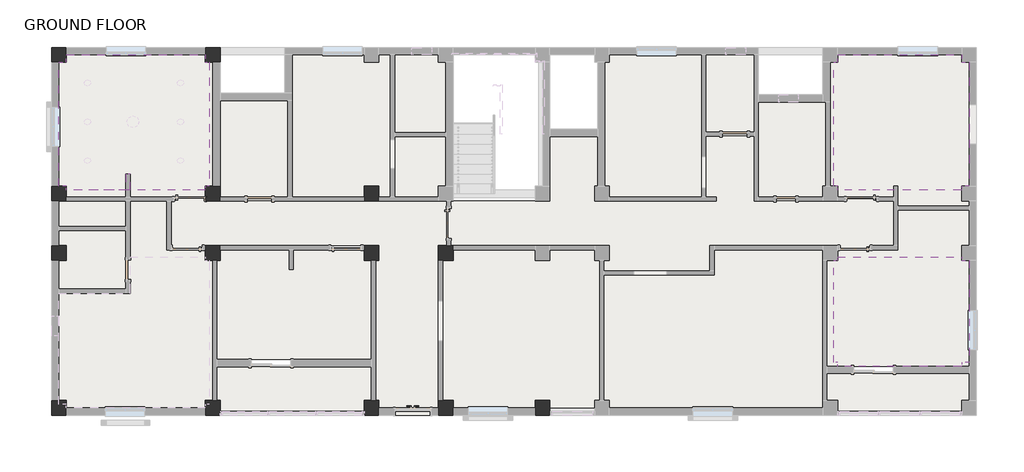
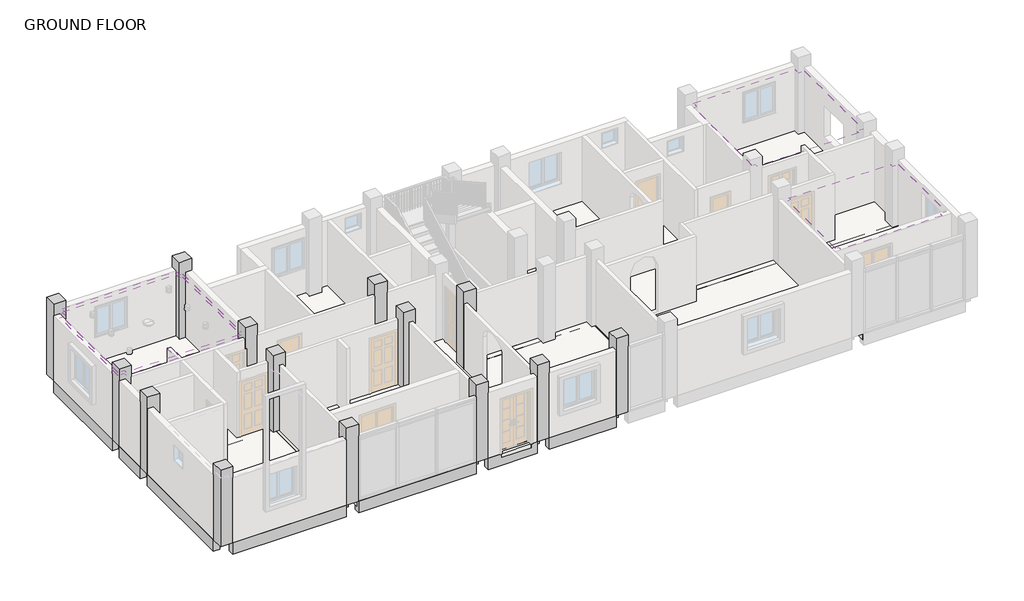
# One storey, part 3 of 5: 21 beams, 14 columns, 4 coverings, 4 slabs.
"""IFC4 building model written with IfcOpenShell, lengths in millimetres."""

from ifc_helpers import new_model, si_unit, point, frame, frame_2d, origin, place, context, project, spatial, polyline, circle_curve, trimmed, segment, composite_curve, outline, extrude, faceted_brep, element, save

model = new_model("IFC4")

# Units and contexts
model_context = context("Model", 3, world=origin())
ifc_project = project(units=[si_unit("LENGTHUNIT", "METRE", prefix="MILLI")], contexts=[model_context])

# Site, building, storey
site = spatial("IfcSite", under=ifc_project)
building = spatial("IfcBuilding", under=site)
storey = spatial("IfcBuildingStorey", under=building, Name="GROUND FLOOR", Elevation=304.8)

# Beams
placement = place(None, origin())
element("IfcBeam", 1, ObjectType="Concrete-Rectangular Beam : 9\" X 18\" BEAM", at=placement, inside=storey, context=model_context, shape_type="SweptSolid", body=[
    extrude(outline(polyline([(-10649.5456086, -10887.8679047), (-10649.5456086, -11116.4679047), (-14916.7456086, -11116.4679047), (-14916.7456086, -10887.8679047), (-10649.5456086, -10887.8679047)])), frame((0.0, 0.0, -152.4), z_axis=(0.0, 0.0, 1.0), x_axis=(1.0, 0.0, 0.0)), (0.0, 0.0, 1.0), 457.2),
])
element("IfcBeam", 2, ObjectType="Concrete-Rectangular Beam : 9\" X 18\" BEAM", at=placement, inside=storey, context=model_context, shape_type="SweptSolid", body=[
    extrude(outline(polyline([(-5772.7456086, -10887.8679047), (-5772.7456086, -11116.4679047), (-10192.3456086, -11116.4679047), (-10192.3456086, -10887.8679047), (-5772.7456086, -10887.8679047)])), frame((0.0, 0.0, -152.4), z_axis=(0.0, 0.0, 1.0), x_axis=(1.0, 0.0, 0.0)), (0.0, 0.0, 1.0), 457.2),
])
element("IfcBeam", 3, ObjectType="Concrete-Rectangular Beam : 9\" X 18\" BEAM", at=placement, inside=storey, context=model_context, shape_type="Brep", body=[
    faceted_brep([(-5315.5456086, -10887.8679047, 304.8), (-5315.5456086, -11116.4679047, 304.8), (-4807.5456086, -11116.4679047, 304.8), (-4807.5456086, -10887.8679047, 304.8), (-5315.5456086, -11116.4679047, -152.4), (-3486.7456086, -11116.4679047, -152.4), (-3486.7456086, -11116.4679047, 304.8), (-3715.3456086, -11116.4679047, 304.8), (-3715.3456086, -11116.4679047, 152.4), (-4807.5456086, -11116.4679047, 152.4), (-5315.5456086, -10887.8679047, -152.4), (-3486.7456086, -10887.8679047, -152.4), (-5315.5456086, -10887.8679047, 152.4), (-4807.5456086, -10887.8679047, 152.4), (-3715.3456086, -10887.8679047, 152.4), (-3715.3456086, -10887.8679047, 304.8), (-3486.7456086, -10887.8679047, 304.8), (-3486.7456086, -10887.8679047, 152.4)], [[[0, 1, 2, 3]], [[4, 5, 6, 7, 8, 9, 2, 1]], [[5, 4, 10, 11]], [[11, 10, 12, 0, 3, 13, 14, 15, 16, 17]], [[16, 6, 5, 11, 17]], [[10, 4, 1, 0, 12]], [[8, 14, 13, 9]], [[14, 8, 7, 15]], [[9, 13, 3, 2]], [[6, 16, 15, 7]]]),
])
element("IfcBeam", 4, ObjectType="Concrete-Rectangular Beam : 9\" X 18\" BEAM", at=placement, inside=storey, context=model_context, shape_type="SweptSolid", body=[
    extrude(outline(polyline([(-518.4083398, -10887.8679047), (-518.4083398, -11116.4679047), (-3029.5456086, -11116.4679047), (-3029.5456086, -10887.8679047), (-518.4083398, -10887.8679047)])), frame((0.0, 0.0, -152.4), z_axis=(0.0, 0.0, 1.0), x_axis=(1.0, 0.0, 0.0)), (0.0, 0.0, 1.0), 457.2),
])
element("IfcBeam", 5, ObjectType="Concrete-Rectangular Beam : 9\" X 18\" BEAM", at=placement, inside=storey, context=model_context, shape_type="SweptSolid", body=[
    extrude(outline(polyline([(-15145.3456086, -4072.3794704), (-15373.9456086, -4072.3794704), (-15373.9456086, -262.3794704), (-15145.3456086, -262.3794704), (-15145.3456086, -4072.3794704)])), frame((0.0, 0.0, -152.4), z_axis=(0.0, 0.0, 1.0), x_axis=(1.0, 0.0, 0.0)), (0.0, 0.0, 1.0), 457.2),
])
element("IfcBeam", 6, ObjectType="Concrete-Rectangular Beam : 9\" X 18\" BEAM", at=placement, inside=storey, context=model_context, shape_type="SweptSolid", body=[
    extrude(outline(polyline([(-15145.3456086, -5901.1794704), (-15373.9456086, -5901.1794704), (-15373.9456086, -4529.5794704), (-15145.3456086, -4529.5794704), (-15145.3456086, -5901.1794704)])), frame((0.0, 0.0, -152.4), z_axis=(0.0, 0.0, 1.0), x_axis=(1.0, 0.0, 0.0)), (0.0, 0.0, 1.0), 457.2),
])
element("IfcBeam", 7, ObjectType="Concrete-Rectangular Beam : 9\" X 18\" BEAM", at=placement, inside=storey, context=model_context, shape_type="SweptSolid", body=[
    extrude(outline(polyline([(-15145.3456086, -10659.2679047), (-15373.9456086, -10659.2679047), (-15373.9456086, -6358.3794704), (-15145.3456086, -6358.3794704), (-15145.3456086, -10659.2679047)])), frame((0.0, 0.0, -152.4), z_axis=(0.0, 0.0, 1.0), x_axis=(1.0, 0.0, 0.0)), (0.0, 0.0, 1.0), 457.2),
])
element("IfcBeam", 8, ObjectType="Concrete-Rectangular Beam : 9\" X 18\" BEAM", at=placement, inside=storey, context=model_context, shape_type="Brep", body=[
    faceted_brep([(-10649.5456086, -4186.6794704, 304.8), (-14916.7456086, -4186.6794704, 304.8), (-14916.7456086, -4415.2794704, 304.8), (-11589.3456086, -4415.2794704, 304.8), (-11589.3456086, -4402.5794704, 304.8), (-10674.9456086, -4402.5794704, 304.8), (-10674.9456086, -4415.2794704, 304.8), (-10649.5456086, -4415.2794704, 304.8), (-14916.7456086, -4415.2794704, -152.4), (-10649.5456086, -4415.2794704, -152.4), (-10674.9456086, -4415.2794704, 152.4), (-11589.3456086, -4415.2794704, 152.4), (-14916.7456086, -4186.6794704, -152.4), (-10649.5456086, -4186.6794704, -152.4), (-10674.9456086, -4402.5794704, 152.4), (-11589.3456086, -4402.5794704, 152.4)], [[[0, 1, 2, 3, 4, 5, 6, 7]], [[8, 9, 7, 6, 10, 11, 3, 2]], [[9, 8, 12, 13]], [[1, 0, 13, 12]], [[1, 12, 8, 2]], [[0, 7, 9, 13]], [[14, 15, 11, 10]], [[15, 4, 3, 11]], [[15, 14, 5, 4]], [[5, 14, 10, 6]]]),
])
element("IfcBeam", 9, ObjectType="Concrete-Rectangular Beam : 9\" X 18\" BEAM", at=placement, inside=storey, context=model_context, shape_type="SweptSolid", body=[
    extrude(outline(polyline([(-5772.7456086, -4186.6794704), (-5772.7456086, -4415.2794704), (-10192.3456086, -4415.2794704), (-10192.3456086, -4186.6794704), (-5772.7456086, -4186.6794704)])), frame((0.0, 0.0, -152.4), z_axis=(0.0, 0.0, 1.0), x_axis=(1.0, 0.0, 0.0)), (0.0, 0.0, 1.0), 457.2),
])
element("IfcBeam", 10, ObjectType="Concrete-Rectangular Beam : 9\" X 18\" BEAM", at=placement, inside=storey, context=model_context, shape_type="SweptSolid", body=[
    extrude(outline(polyline([(-3486.7456086, -4186.6794704), (-3486.7456086, -4415.2794704), (-5315.5456086, -4415.2794704), (-5315.5456086, -4186.6794704), (-3486.7456086, -4186.6794704)])), frame((0.0, 0.0, -152.4), z_axis=(0.0, 0.0, 1.0), x_axis=(1.0, 0.0, 0.0)), (0.0, 0.0, 1.0), 457.2),
])
element("IfcBeam", 11, ObjectType="Concrete-Rectangular Beam : 9\" X 18\" BEAM", at=placement, inside=storey, context=model_context, shape_type="SweptSolid", body=[
    extrude(outline(polyline([(-10306.6456086, -4072.3794704), (-10535.2456086, -4072.3794704), (-10535.2456086, -262.3794704), (-10306.6456086, -262.3794704), (-10306.6456086, -4072.3794704)])), frame((0.0, 0.0, -152.4), z_axis=(0.0, 0.0, 1.0), x_axis=(1.0, 0.0, 0.0)), (0.0, 0.0, 1.0), 457.2),
])
element("IfcBeam", 12, ObjectType="Concrete-Rectangular Beam : 9\" X 18\" BEAM", at=placement, inside=storey, context=model_context, shape_type="SweptSolid", body=[
    extrude(outline(polyline([(-10649.5456086, -6015.4794704), (-10649.5456086, -6244.0794704), (-14916.7456086, -6244.0794704), (-14916.7456086, -6015.4794704), (-10649.5456086, -6015.4794704)])), frame((0.0, 0.0, -152.4), z_axis=(0.0, 0.0, 1.0), x_axis=(1.0, 0.0, 0.0)), (0.0, 0.0, 1.0), 457.2),
])
element("IfcBeam", 13, ObjectType="Concrete-Rectangular Beam : 9\" X 18\" BEAM", at=placement, inside=storey, context=model_context, shape_type="SweptSolid", body=[
    extrude(outline(polyline([(-5772.7456086, -6015.4794704), (-5772.7456086, -6244.0794704), (-10192.3456086, -6244.0794704), (-10192.3456086, -6015.4794704), (-5772.7456086, -6015.4794704)])), frame((0.0, 0.0, -152.4), z_axis=(0.0, 0.0, 1.0), x_axis=(1.0, 0.0, 0.0)), (0.0, 0.0, 1.0), 457.2),
])
element("IfcBeam", 14, ObjectType="Concrete-Rectangular Beam : 9\" X 18\" BEAM", at=placement, inside=storey, context=model_context, shape_type="SweptSolid", body=[
    extrude(outline(polyline([(-3486.7456086, -6244.0794704), (-5315.5456086, -6244.0794704), (-5315.5456086, -6015.4794704), (-3486.7456086, -6015.4794704), (-3486.7456086, -6244.0794704)])), frame((0.0, 0.0, -152.4), z_axis=(0.0, 0.0, 1.0), x_axis=(1.0, 0.0, 0.0)), (0.0, 0.0, 1.0), 304.8),
])
element("IfcBeam", 15, ObjectType="Concrete-Rectangular Beam : 9\" X 18\" BEAM", at=placement, inside=storey, context=model_context, shape_type="SweptSolid", body=[
    extrude(outline(polyline([(-3029.5456086, -6244.0794704), (-3029.5456086, -6015.4794704), (-518.4083398, -6015.4794704), (-518.4083398, -6244.0794704), (-3029.5456086, -6244.0794704)])), frame((0.0, 0.0, -152.4), z_axis=(0.0, 0.0, 1.0), x_axis=(1.0, 0.0, 0.0)), (0.0, 0.0, 1.0), 457.2),
])
element("IfcBeam", 16, ObjectType="Concrete-Rectangular Beam : 9\" X 18\" BEAM", at=placement, inside=storey, context=model_context, shape_type="SweptSolid", body=[
    extrude(outline(polyline([(-10535.2456086, -6358.3794704), (-10306.6456086, -6358.3794704), (-10306.6456086, -10659.2679047), (-10535.2456086, -10659.2679047), (-10535.2456086, -6358.3794704)])), frame((0.0, 0.0, -152.4), z_axis=(0.0, 0.0, 1.0), x_axis=(1.0, 0.0, 0.0)), (0.0, 0.0, 1.0), 457.2),
])
element("IfcBeam", 17, ObjectType="Concrete-Rectangular Beam : 9\" X 18\" BEAM", at=placement, inside=storey, context=model_context, shape_type="SweptSolid", body=[
    extrude(outline(polyline([(-5658.4456086, -6358.3794704), (-5429.8456086, -6358.3794704), (-5429.8456086, -10659.2679047), (-5658.4456086, -10659.2679047), (-5658.4456086, -6358.3794704)])), frame((0.0, 0.0, -152.4), z_axis=(0.0, 0.0, 1.0), x_axis=(1.0, 0.0, 0.0)), (0.0, 0.0, 1.0), 457.2),
])
element("IfcBeam", 18, ObjectType="Concrete-Rectangular Beam : 9\" X 18\" BEAM", at=placement, inside=storey, context=model_context, shape_type="SweptSolid", body=[
    extrude(outline(polyline([(-3372.4456086, -6358.3794704), (-3143.8456086, -6358.3794704), (-3143.8456086, -10659.2679047), (-3372.4456086, -10659.2679047), (-3372.4456086, -6358.3794704)])), frame((0.0, 0.0, -152.4), z_axis=(0.0, 0.0, 1.0), x_axis=(1.0, 0.0, 0.0)), (0.0, 0.0, 1.0), 457.2),
])
element("IfcBeam", 19, ObjectType="Concrete-Rectangular Beam : 9\" X 18\" BEAM", at=placement, inside=storey, context=model_context, shape_type="SweptSolid", body=[
    extrude(outline(polyline([(-404.1083398, -6358.3794704), (-175.5083398, -6358.3794704), (-175.5083398, -10659.2679047), (-404.1083398, -10659.2679047), (-404.1083398, -6358.3794704)])), frame((0.0, 0.0, -152.4), z_axis=(0.0, 0.0, 1.0), x_axis=(1.0, 0.0, 0.0)), (0.0, 0.0, 1.0), 457.2),
])
element("IfcBeam", 20, ObjectType="Concrete-Rectangular Beam : 9\" X 18\" BEAM", at=placement, inside=storey, context=model_context, shape_type="SweptSolid", body=[
    extrude(outline(polyline([(-5658.4456086, -5901.1794704), (-5658.4456086, -4529.5794704), (-5429.8456086, -4529.5794704), (-5429.8456086, -5901.1794704), (-5658.4456086, -5901.1794704)])), frame((0.0, 0.0, -152.4), z_axis=(0.0, 0.0, 1.0), x_axis=(1.0, 0.0, 0.0)), (0.0, 0.0, 1.0), 304.8),
])
element("IfcBeam", 21, ObjectType="Concrete-Rectangular Beam : 9\" X 18\" BEAM", at=placement, inside=storey, context=model_context, shape_type="SweptSolid", body=[
    extrude(outline(polyline([(-10535.2456086, -5901.1794704), (-10535.2456086, -4529.5794704), (-10306.6456086, -4529.5794704), (-10306.6456086, -5901.1794704), (-10535.2456086, -5901.1794704)])), frame((0.0, 0.0, -152.4), z_axis=(0.0, 0.0, 1.0), x_axis=(1.0, 0.0, 0.0)), (0.0, 0.0, 1.0), 304.8),
])

# Columns
element("IfcColumn", 22, ObjectType="Concrete-Rectangular-Column : COLUMN 18\" X 18\"", at=placement, inside=storey, context=model_context, shape_type="SweptSolid", body=[
    extrude(outline(polyline([(-14916.7456086, 194.8205296), (-14916.7456086, -262.3794704), (-15373.9456086, -262.3794704), (-15373.9456086, 194.8205296), (-14916.7456086, 194.8205296)])), frame((0.0, 0.0, 304.8), z_axis=(0.0, 0.0, 1.0), x_axis=(1.0, 0.0, 0.0)), (0.0, 0.0, 1.0), 3048.0),
])
element("IfcColumn", 23, ObjectType="Concrete-Rectangular-Column : COLUMN 18\" X 18\"", at=placement, inside=storey, context=model_context, shape_type="SweptSolid", body=[
    extrude(outline(polyline([(-10192.3456086, 194.8205296), (-10192.3456086, -262.3794704), (-10649.5456086, -262.3794704), (-10649.5456086, 194.8205296), (-10192.3456086, 194.8205296)])), frame((0.0, 0.0, 304.8), z_axis=(0.0, 0.0, 1.0), x_axis=(1.0, 0.0, 0.0)), (0.0, 0.0, 1.0), 3048.0),
])
element("IfcColumn", 24, ObjectType="Concrete-Rectangular-Column : COLUMN 18\" X 18\"", at=placement, inside=storey, context=model_context, shape_type="SweptSolid", body=[
    extrude(outline(polyline([(-61.2083398, -10659.2679047), (-61.2083398, -11116.4679047), (-518.4083398, -11116.4679047), (-518.4083398, -10659.2679047), (-61.2083398, -10659.2679047)])), frame((0.0, 0.0, 304.8), z_axis=(0.0, 0.0, 1.0), x_axis=(1.0, 0.0, 0.0)), (0.0, 0.0, 1.0), 3048.0),
])
element("IfcColumn", 25, ObjectType="Concrete-Rectangular-Column : COLUMN 18\" X 18\"", at=placement, inside=storey, context=model_context, shape_type="SweptSolid", body=[
    extrude(outline(polyline([(-3029.5456086, -10659.2679047), (-3029.5456086, -11116.4679047), (-3486.7456086, -11116.4679047), (-3486.7456086, -10659.2679047), (-3029.5456086, -10659.2679047)])), frame((0.0, 0.0, 304.8), z_axis=(0.0, 0.0, 1.0), x_axis=(1.0, 0.0, 0.0)), (0.0, 0.0, 1.0), 3048.0),
])
element("IfcColumn", 26, ObjectType="Concrete-Rectangular-Column : COLUMN 18\" X 18\"", at=placement, inside=storey, context=model_context, shape_type="SweptSolid", body=[
    extrude(outline(polyline([(-5315.5456086, -10659.2679047), (-5315.5456086, -11116.4679047), (-5772.7456086, -11116.4679047), (-5772.7456086, -10659.2679047), (-5315.5456086, -10659.2679047)])), frame((0.0, 0.0, 304.8), z_axis=(0.0, 0.0, 1.0), x_axis=(1.0, 0.0, 0.0)), (0.0, 0.0, 1.0), 3048.0),
])
element("IfcColumn", 27, ObjectType="Concrete-Rectangular-Column : COLUMN 18\" X 18\"", at=placement, inside=storey, context=model_context, shape_type="SweptSolid", body=[
    extrude(outline(polyline([(-10192.3456086, -10659.2679047), (-10192.3456086, -11116.4679047), (-10649.5456086, -11116.4679047), (-10649.5456086, -10659.2679047), (-10192.3456086, -10659.2679047)])), frame((0.0, 0.0, 304.8), z_axis=(0.0, 0.0, 1.0), x_axis=(1.0, 0.0, 0.0)), (0.0, 0.0, 1.0), 3048.0),
])
element("IfcColumn", 28, ObjectType="Concrete-Rectangular-Column : COLUMN 18\" X 18\"", at=placement, inside=storey, context=model_context, shape_type="SweptSolid", body=[
    extrude(outline(polyline([(-14916.7456086, -10659.2679047), (-14916.7456086, -11116.4679047), (-15373.9456086, -11116.4679047), (-15373.9456086, -10659.2679047), (-14916.7456086, -10659.2679047)])), frame((0.0, 0.0, 304.8), z_axis=(0.0, 0.0, 1.0), x_axis=(1.0, 0.0, 0.0)), (0.0, 0.0, 1.0), 3048.0),
])
element("IfcColumn", 29, ObjectType="Concrete-Rectangular-Column : COLUMN 18\" X 18\"", at=placement, inside=storey, context=model_context, shape_type="SweptSolid", body=[
    extrude(outline(polyline([(-14916.7456086, -5901.1794704), (-14916.7456086, -6358.3794704), (-15373.9456086, -6358.3794704), (-15373.9456086, -5901.1794704), (-14916.7456086, -5901.1794704)])), frame((0.0, 0.0, 304.8), z_axis=(0.0, 0.0, 1.0), x_axis=(1.0, 0.0, 0.0)), (0.0, 0.0, 1.0), 3048.0),
])
element("IfcColumn", 30, ObjectType="Concrete-Rectangular-Column : COLUMN 18\" X 18\"", at=placement, inside=storey, context=model_context, shape_type="SweptSolid", body=[
    extrude(outline(polyline([(-14916.7456086, -4072.3794704), (-14916.7456086, -4529.5794704), (-15373.9456086, -4529.5794704), (-15373.9456086, -4072.3794704), (-14916.7456086, -4072.3794704)])), frame((0.0, 0.0, 304.8), z_axis=(0.0, 0.0, 1.0), x_axis=(1.0, 0.0, 0.0)), (0.0, 0.0, 1.0), 3048.0),
])
element("IfcColumn", 31, ObjectType="Concrete-Rectangular-Column : COLUMN 18\" X 18\"", at=placement, inside=storey, context=model_context, shape_type="SweptSolid", body=[
    extrude(outline(polyline([(-10192.3456086, -4072.3794704), (-10192.3456086, -4529.5794704), (-10649.5456086, -4529.5794704), (-10649.5456086, -4072.3794704), (-10192.3456086, -4072.3794704)])), frame((0.0, 0.0, 304.8), z_axis=(0.0, 0.0, 1.0), x_axis=(1.0, 0.0, 0.0)), (0.0, 0.0, 1.0), 3048.0),
])
element("IfcColumn", 32, ObjectType="Concrete-Rectangular-Column : COLUMN 18\" X 18\"", at=placement, inside=storey, context=model_context, shape_type="SweptSolid", body=[
    extrude(outline(polyline([(-5315.5456086, -4072.3794704), (-5315.5456086, -4529.5794704), (-5772.7456086, -4529.5794704), (-5772.7456086, -4072.3794704), (-5315.5456086, -4072.3794704)])), frame((0.0, 0.0, 304.8), z_axis=(0.0, 0.0, 1.0), x_axis=(1.0, 0.0, 0.0)), (0.0, 0.0, 1.0), 3048.0),
])
element("IfcColumn", 33, ObjectType="Concrete-Rectangular-Column : COLUMN 18\" X 18\"", at=placement, inside=storey, context=model_context, shape_type="SweptSolid", body=[
    extrude(outline(polyline([(-3029.5456086, -5901.1794704), (-3029.5456086, -6358.3794704), (-3486.7456086, -6358.3794704), (-3486.7456086, -5901.1794704), (-3029.5456086, -5901.1794704)])), frame((0.0, 0.0, 304.8), z_axis=(0.0, 0.0, 1.0), x_axis=(1.0, 0.0, 0.0)), (0.0, 0.0, 1.0), 3048.0),
])
element("IfcColumn", 34, ObjectType="Concrete-Rectangular-Column : COLUMN 18\" X 18\"", at=placement, inside=storey, context=model_context, shape_type="SweptSolid", body=[
    extrude(outline(polyline([(-5315.5456086, -5901.1794704), (-5315.5456086, -6358.3794704), (-5772.7456086, -6358.3794704), (-5772.7456086, -5901.1794704), (-5315.5456086, -5901.1794704)])), frame((0.0, 0.0, 304.8), z_axis=(0.0, 0.0, 1.0), x_axis=(1.0, 0.0, 0.0)), (0.0, 0.0, 1.0), 3048.0),
])
element("IfcColumn", 35, ObjectType="Concrete-Rectangular-Column : COLUMN 18\" X 18\"", at=placement, inside=storey, context=model_context, shape_type="SweptSolid", body=[
    extrude(outline(polyline([(-10192.3456086, -5901.1794704), (-10192.3456086, -6358.3794704), (-10649.5456086, -6358.3794704), (-10649.5456086, -5901.1794704), (-10192.3456086, -5901.1794704)])), frame((0.0, 0.0, 304.8), z_axis=(0.0, 0.0, 1.0), x_axis=(1.0, 0.0, 0.0)), (0.0, 0.0, 1.0), 3048.0),
])

# Coverings
element("IfcCovering", 36, ObjectType="GWB on Mtl. Stud", at=placement, inside=storey, context=model_context, shape_type="SweptSolid", body=[
    extrude(outline(polyline([(-14916.7456086, -262.3794704), (-14916.7456086, -33.7794704), (-10649.5456086, -33.7794704), (-10649.5456086, -262.3794704), (-10535.2456086, -262.3794704), (-10535.2456086, -4072.3794704), (-10649.5456086, -4072.3794704), (-10649.5456086, -4186.6794704), (-12959.7401855, -4186.6794704), (-12959.7401855, -3705.5659448), (-13086.7401855, -3705.5659448), (-13086.7401855, -4186.6794704), (-14916.7456086, -4186.6794704), (-14916.7456086, -4072.3794704), (-15145.3456086, -4072.3794704), (-15145.3456086, -262.3794704), (-14916.7456086, -262.3794704)]), holes=[composite_curve([segment(trimmed(circle_curve(frame_2d((-14269.0456086, -897.3794704)), 76.2), [point((-14345.2456086, -897.3794704))], [point((-14192.8456086, -897.3794704))], True, "CARTESIAN"), True, "CONTINUOUS"), segment(trimmed(circle_curve(frame_2d((-14269.0456086, -897.3794704)), 76.2), [point((-14192.8456086, -897.3794704))], [point((-14345.2456086, -897.3794704))], True, "CARTESIAN"), True, "CONTINUOUS")], self_intersect=False), composite_curve([segment(trimmed(circle_curve(frame_2d((-14269.0456086, -3284.9794704)), 76.2), [point((-14345.2456086, -3284.9794704))], [point((-14192.8456086, -3284.9794704))], True, "CARTESIAN"), True, "CONTINUOUS"), segment(trimmed(circle_curve(frame_2d((-14269.0456086, -3284.9794704)), 76.2), [point((-14192.8456086, -3284.9794704))], [point((-14345.2456086, -3284.9794704))], True, "CARTESIAN"), True, "CONTINUOUS")], self_intersect=False), composite_curve([segment(trimmed(circle_curve(frame_2d((-14269.0456086, -2091.1794704)), 76.2), [point((-14345.2456086, -2091.1794704))], [point((-14192.8456086, -2091.1794704))], True, "CARTESIAN"), True, "CONTINUOUS"), segment(trimmed(circle_curve(frame_2d((-14269.0456086, -2091.1794704)), 76.2), [point((-14192.8456086, -2091.1794704))], [point((-14345.2456086, -2091.1794704))], True, "CARTESIAN"), True, "CONTINUOUS")], self_intersect=False), composite_curve([segment(trimmed(circle_curve(frame_2d((-11411.5456086, -897.3794704)), 76.2), [point((-11335.3456086, -897.3794704))], [point((-11487.7456086, -897.3794704))], True, "CARTESIAN"), True, "CONTINUOUS"), segment(trimmed(circle_curve(frame_2d((-11411.5456086, -897.3794704)), 76.2), [point((-11487.7456086, -897.3794704))], [point((-11335.3456086, -897.3794704))], True, "CARTESIAN"), True, "CONTINUOUS")], self_intersect=False), composite_curve([segment(trimmed(circle_curve(frame_2d((-11411.5456086, -3284.9794704)), 76.2), [point((-11335.3456086, -3284.9794704))], [point((-11487.7456086, -3284.9794704))], True, "CARTESIAN"), True, "CONTINUOUS"), segment(trimmed(circle_curve(frame_2d((-11411.5456086, -3284.9794704)), 76.2), [point((-11487.7456086, -3284.9794704))], [point((-11335.3456086, -3284.9794704))], True, "CARTESIAN"), True, "CONTINUOUS")], self_intersect=False), composite_curve([segment(trimmed(circle_curve(frame_2d((-11411.5456086, -2091.1794704)), 76.2), [point((-11335.3456086, -2091.1794704))], [point((-11487.7456086, -2091.1794704))], True, "CARTESIAN"), True, "CONTINUOUS"), segment(trimmed(circle_curve(frame_2d((-11411.5456086, -2091.1794704)), 76.2), [point((-11487.7456086, -2091.1794704))], [point((-11335.3456086, -2091.1794704))], True, "CARTESIAN"), True, "CONTINUOUS")], self_intersect=False)]), frame((0.0, 0.0, 2870.2), z_axis=(0.0, 0.0, 1.0), x_axis=(1.0, 0.0, 0.0)), (0.0, 0.0, 1.0), 107.95),
])
element("IfcCovering", 37, ObjectType="GWB on Mtl. Stud", at=placement, inside=storey, context=model_context, shape_type="SweptSolid", body=[
    extrude(outline(polyline([(-15145.3456086, -4072.3794704), (-15145.3456086, -262.3794704), (-14916.7456086, -262.3794704), (-14916.7456086, -33.7794704), (-10649.5456086, -33.7794704), (-10649.5456086, -262.3794704), (-10535.2456086, -262.3794704), (-10535.2456086, -4072.3794704), (-10649.5456086, -4072.3794704), (-10649.5456086, -4186.6794704), (-12959.7401855, -4186.6794704), (-14916.7456086, -4186.6794704), (-14916.7456086, -4072.3794704), (-15145.3456086, -4072.3794704)]), holes=[polyline([(-14840.5456086, -3881.8794704), (-10840.0456086, -3881.8794704), (-10840.0456086, -338.5794704), (-14840.5456086, -338.5794704), (-14840.5456086, -3881.8794704)])]), frame((0.0, 0.0, 2743.2), z_axis=(0.0, 0.0, 1.0), x_axis=(1.0, 0.0, 0.0)), (0.0, 0.0, 1.0), 107.95),
    extrude(outline(polyline([(-14688.1456086, -3729.4794704), (-14688.1456086, -490.9794704), (-10992.4456086, -490.9794704), (-10992.4456086, -3729.4794704), (-14688.1456086, -3729.4794704)]), holes=[polyline([(-11144.8456086, -643.3794704), (-14535.7456086, -643.3794704), (-14535.7456086, -3577.0794704), (-11144.8456086, -3577.0794704), (-11144.8456086, -643.3794704)])]), frame((0.0, 0.0, 2743.2), z_axis=(0.0, 0.0, 1.0), x_axis=(1.0, 0.0, 0.0)), (0.0, 0.0, 1.0), 107.95),
])
element("IfcCovering", 38, ObjectType="GWB on Mtl. Stud", at=placement, inside=storey, context=model_context, shape_type="SweptSolid", body=[
    extrude(outline(polyline([(8991.0043914, -3729.4794704), (8991.0043914, -490.9794704), (12477.1543914, -490.9794704), (12477.1543914, -3729.4794704), (8991.0043914, -3729.4794704)]), holes=[polyline([(12324.7543914, -643.3794704), (9162.4543914, -643.3794704), (9162.4543914, -3577.0794704), (12324.7543914, -3577.0794704), (12324.7543914, -643.3794704)])]), frame((0.0, 0.0, 2743.2), z_axis=(0.0, 0.0, 1.0), x_axis=(1.0, 0.0, 0.0)), (0.0, 0.0, 1.0), 107.95),
    extrude(outline(polyline([(8660.1098601, -4072.3794704), (8660.1098601, -262.3794704), (8774.4128058, -262.3794704), (8774.4128058, -33.7794704), (12584.4128058, -33.7794704), (12584.4128058, -262.3794704), (12813.0098601, -262.3794704), (12813.0098601, -4072.3794704), (12584.4128058, -4072.3794704), (12584.4128058, -4186.6794704), (10509.8598145, -4186.6794704), (8774.4128058, -4186.6794704), (8774.4128058, -4072.3794704), (8660.1098601, -4072.3794704)]), holes=[polyline([(8838.6043914, -338.5794704), (8838.6043914, -3881.8794704), (12629.5543914, -3881.8794704), (12629.5543914, -338.5794704), (8838.6043914, -338.5794704)])]), frame((0.0, 0.0, 2743.2), z_axis=(0.0, 0.0, 1.0), x_axis=(1.0, 0.0, 0.0)), (0.0, 0.0, 1.0), 107.95),
])
element("IfcCovering", 39, ObjectType="GWB on Mtl. Stud", at=placement, inside=storey, context=model_context, shape_type="SweptSolid", body=[
    extrude(outline(polyline([(8991.0043914, -9147.9642361), (8991.0043914, -6726.6794704), (12477.1543914, -6726.6794704), (12477.1543914, -9147.9642361), (8991.0043914, -9147.9642361)]), holes=[polyline([(12324.7543914, -7031.4298611), (9162.4543914, -7031.4298611), (9162.4543914, -8995.5642361), (12324.7543914, -8995.5642361), (12324.7543914, -7031.4298611)])]), frame((0.0, 0.0, 2743.2), z_axis=(0.0, 0.0, 1.0), x_axis=(1.0, 0.0, 0.0)), (0.0, 0.0, 1.0), 107.95),
    extrude(outline(polyline([(8660.1098601, -9490.8642361), (8660.1098601, -6358.3685356), (8774.4128058, -6358.3685356), (8774.4128058, -6244.0794704), (12584.4128058, -6244.0794704), (12584.4128058, -6358.3794704), (12813.0098601, -6358.3794704), (12813.0098601, -9490.8642361), (12584.4128058, -9490.8642361), (12584.4128058, -9605.1642361), (10509.8598145, -9605.1642361), (8774.4128058, -9605.1642361), (8774.4128058, -9490.8642361), (8660.1098601, -9490.8642361)]), holes=[polyline([(12629.5543914, -6498.0794704), (8838.6043914, -6498.0794704), (8838.6043914, -9300.3642361), (12629.5543914, -9300.3642361), (12629.5543914, -6498.0794704)])]), frame((0.0, 0.0, 2743.2), z_axis=(0.0, 0.0, 1.0), x_axis=(1.0, 0.0, 0.0)), (0.0, 0.0, 1.0), 107.95),
])

# Slabs
element("IfcSlab", 40, ObjectType="MARBLE FLOORING 6\"", at=placement, inside=storey, context=model_context, shape_type="SweptSolid", body=[
    extrude(outline(polyline([(-13086.7401855, -4529.5794704), (-13086.7401855, -5304.2794704), (-15145.3456086, -5304.2794704), (-15145.3456086, -4529.5794704), (-13086.7401855, -4529.5794704)])), frame((0.0, 0.0, 152.4), z_axis=(0.0, 0.0, 1.0), x_axis=(1.0, 0.0, 0.0)), (0.0, 0.0, 1.0), 152.4),
    extrude(outline(polyline([(-13086.7401855, -5431.2794704), (-13086.7401855, -6334.4659448), (-13023.2401855, -6334.4659448), (-13023.2401855, -6944.0659448), (-13086.7401855, -6944.0659448), (-13086.7401855, -7236.1659448), (-15145.3456086, -7236.1659448), (-15145.3456086, -6358.3794704), (-14916.7456086, -6358.3794704), (-14916.7456086, -5901.1794704), (-15145.3456086, -5901.1794704), (-15145.3456086, -5431.2794704), (-13086.7401855, -5431.2794704)])), frame((0.0, 0.0, 152.4), z_axis=(0.0, 0.0, 1.0), x_axis=(1.0, 0.0, 0.0)), (0.0, 0.0, 1.0), 152.4),
    extrude(outline(polyline([(-8109.5456086, -1443.4794704), (-8109.5456086, -4402.5794704), (-8603.1541526, -4402.5794704), (-8603.1541526, -4529.5794704), (-9366.8456086, -4529.5794704), (-9366.8456086, -4402.5794704), (-10192.3456086, -4402.5794704), (-10192.3456086, -1443.4794704), (-8109.5456086, -1443.4794704)])), frame((0.0, 0.0, 152.4), z_axis=(0.0, 0.0, 1.0), x_axis=(1.0, 0.0, 0.0)), (0.0, 0.0, 1.0), 152.4),
    extrude(outline(polyline([(-3486.7456086, -33.7794704), (-3486.7456086, -262.3794704), (-3258.1456086, -262.3794704), (-3258.1456086, -2421.3794704), (-4832.9456086, -2421.3794704), (-4832.9456086, -33.7794704), (-3486.7456086, -33.7794704)])), frame((0.0, 0.0, 152.4), z_axis=(0.0, 0.0, 1.0), x_axis=(1.0, 0.0, 0.0)), (0.0, 0.0, 1.0), 152.4),
    extrude(outline(polyline([(6212.5916602, -33.7794704), (6212.5916602, -2408.6794704), (5996.6916602, -2408.6794704), (5996.6916602, -2535.6794704), (5234.6916602, -2535.6794704), (5234.6916602, -2408.6794704), (4726.6916602, -2408.6794704), (4726.6916602, -33.7794704), (6212.5916602, -33.7794704)])), frame((0.0, 0.0, 152.4), z_axis=(0.0, 0.0, 1.0), x_axis=(1.0, 0.0, 0.0)), (0.0, 0.0, 1.0), 152.4),
    extrude(outline(polyline([(8418.8128058, -1481.5794704), (8418.8128058, -4072.3794704), (8317.2128058, -4072.3794704), (8317.2128058, -4402.5794704), (7495.2916602, -4402.5794704), (7495.2916602, -4529.5794704), (6885.6916602, -4529.5794704), (6885.6916602, -4402.5794704), (6339.5916602, -4402.5794704), (6339.5916602, -1481.5794704), (8418.8128058, -1481.5794704)])), frame((0.0, 0.0, 152.4), z_axis=(0.0, 0.0, 1.0), x_axis=(1.0, 0.0, 0.0)), (0.0, 0.0, 1.0), 152.4),
])
element("IfcSlab", 41, ObjectType="Wood Joist 10\" - Ceramic Tile", at=placement, inside=storey, context=model_context, shape_type="SweptSolid", body=[
    extrude(outline(polyline([(-10192.3456086, -10659.2679047), (-10293.9456086, -10659.2679047), (-10293.9456086, -9630.5679047), (-5544.1456086, -9630.5679047), (-5544.1456086, -10659.2679047), (-5772.7456086, -10659.2679047), (-5772.7456086, -10989.4679047), (-10192.3456086, -10989.4679047), (-10192.3456086, -10659.2679047)])), frame((0.0, 0.0, 31.75), z_axis=(0.0, 0.0, 1.0), x_axis=(1.0, 0.0, 0.0)), (0.0, 0.0, 1.0), 273.05),
    extrude(outline(polyline([(8444.2128058, -9833.7679047), (12813.0128058, -9833.7679047), (12813.0128058, -10659.2679047), (12584.4128058, -10659.2679047), (12584.4128058, -11052.9679047), (8774.4128058, -11052.9679047), (8774.4128058, -10659.2679047), (8444.2128058, -10659.2679047), (8444.2128058, -9833.7679047)])), frame((0.0, 0.0, 31.75), z_axis=(0.0, 0.0, 1.0), x_axis=(1.0, 0.0, 0.0)), (0.0, 0.0, 1.0), 273.05),
])
element("IfcSlab", 42, ObjectType="white MARBLE FLOORING 6\" 2", at=placement, inside=storey, context=model_context, shape_type="SweptSolid", body=[
    extrude(outline(polyline([(-12959.7401855, -4402.5794704), (-12959.7401855, -3705.5659448), (-13086.7401855, -3705.5659448), (-13086.7401855, -4402.5794704), (-14916.7456086, -4402.5794704), (-14916.7456086, -4072.3794704), (-15145.3456086, -4072.3794704), (-15145.3456086, -262.3794704), (-14916.7456086, -262.3794704), (-14916.7456086, -33.7794704), (-10649.5456086, -33.7794704), (-10649.5456086, -262.3794704), (-10420.9456086, -262.3794704), (-10420.9456086, -4072.3794704), (-10649.5456086, -4072.3794704), (-10649.5456086, -4402.5794704), (-11589.3456086, -4402.5794704), (-12959.7401855, -4402.5794704)])), frame((0.0, 0.0, 152.4), z_axis=(0.0, 0.0, 1.0), x_axis=(1.0, 0.0, 0.0)), (0.0, 0.0, 1.0), 152.4),
    extrude(outline(polyline([(-15145.3456086, -10659.2679047), (-15145.3456086, -7363.1659448), (-12959.7401855, -7363.1659448), (-12959.7401855, -6944.0659448), (-13023.2401855, -6944.0659448), (-13023.2401855, -6334.4659448), (-12959.7401855, -6334.4659448), (-12959.7401855, -4529.5794704), (-11829.4401855, -4529.5794704), (-11829.4401855, -6028.1794704), (-11690.342897, -6028.1794704), (-11690.342897, -5967.8544704), (-10750.542897, -5967.8544704), (-10750.542897, -6028.1794704), (-10649.5456086, -6028.1794704), (-10649.5456086, -6358.3794704), (-10420.9456086, -6358.3794704), (-10420.9456086, -10659.2679047), (-10649.5456086, -10659.2679047), (-10649.5456086, -10887.8679047), (-14916.7456086, -10887.8679047), (-14916.7456086, -10659.2679047), (-15145.3456086, -10659.2679047)])), frame((0.0, 0.0, 152.4), z_axis=(0.0, 0.0, 1.0), x_axis=(1.0, 0.0, 0.0)), (0.0, 0.0, 1.0), 152.4),
    extrude(outline(polyline([(-5544.1456086, -9401.9679047), (-10293.9456086, -9401.9679047), (-10293.9456086, -6358.3794704), (-10192.3456086, -6358.3794704), (-10192.3456086, -6028.1794704), (-8071.4456086, -6028.1794704), (-8071.4456086, -6637.7794704), (-7944.4456086, -6637.7794704), (-7944.4456086, -6028.1794704), (-6788.7456086, -6028.1794704), (-6788.7456086, -5967.8544704), (-5874.3456086, -5967.8544704), (-5874.3456086, -6028.1794704), (-5772.7456086, -6028.1794704), (-5772.7456086, -6358.3794704), (-5544.1456086, -6358.3794704), (-5544.1456086, -9401.9679047)])), frame((0.0, 0.0, 152.4), z_axis=(0.0, 0.0, 1.0), x_axis=(1.0, 0.0, 0.0)), (0.0, 0.0, 1.0), 152.4),
    extrude(outline(polyline([(-3029.5456086, -10659.2679047), (-3359.7456086, -10659.2679047), (-3359.7456086, -6358.3794704), (-3029.5456086, -6358.3794704), (-3029.5456086, -6028.1794704), (-518.4083398, -6028.1794704), (-518.4083398, -6358.3794704), (-61.2083398, -6358.3794704), (-61.2083398, -6028.1794704), (1310.3916602, -6028.1794704), (1310.3916602, -6358.3794704), (1462.7916602, -6358.3794704), (1462.7916602, -10659.2679047), (1310.3916602, -10659.2679047), (1310.3916602, -10887.8679047), (-61.2083398, -10887.8679047), (-61.2083398, -10659.2679047), (-518.4083398, -10659.2679047), (-518.4083398, -10887.8679047), (-3029.5456086, -10887.8679047), (-3029.5456086, -10659.2679047)])), frame((0.0, 0.0, 152.4), z_axis=(0.0, 0.0, 1.0), x_axis=(1.0, 0.0, 0.0)), (0.0, 0.0, 1.0), 152.4),
    extrude(outline(polyline([(4980.6916602, -6802.8794704), (4980.6916602, -6028.1794704), (8317.2128058, -6028.1794704), (8317.2128058, -10887.8679047), (1767.5916602, -10887.8679047), (1767.5916602, -10659.2679047), (1589.7916602, -10659.2679047), (1589.7916602, -6802.8794704), (4980.6916602, -6802.8794704)])), frame((0.0, 0.0, 152.4), z_axis=(0.0, 0.0, 1.0), x_axis=(1.0, 0.0, 0.0)), (0.0, 0.0, 1.0), 152.4),
    extrude(outline(polyline([(12813.0128058, -9605.1679047), (8444.2128058, -9605.1679047), (8444.2128058, -6358.3794704), (8774.4128058, -6358.3794704), (8774.4128058, -6028.1794704), (8850.6128058, -6028.1794704), (8850.6128058, -5967.8544704), (9765.0128058, -5967.8544704), (9765.0128058, -6028.1794704), (10628.6128058, -6028.1794704), (10628.6128058, -4808.9794704), (12813.0128058, -4808.9794704), (12813.0128058, -5901.1794704), (12584.4128058, -5901.1794704), (12584.4128058, -6358.3794704), (12813.0128058, -6358.3794704), (12813.0128058, -9605.1679047)])), frame((0.0, 0.0, 152.4), z_axis=(0.0, 0.0, 1.0), x_axis=(1.0, 0.0, 0.0)), (0.0, 0.0, 1.0), 152.4),
    extrude(outline(polyline([(12813.0128058, -4681.9794704), (10628.6128058, -4681.9794704), (10628.6128058, -4072.3794704), (10501.6128058, -4072.3794704), (10501.6128058, -4402.5794704), (9968.2128058, -4402.5794704), (9968.2128058, -4466.0794704), (9053.8128058, -4466.0794704), (9053.8128058, -4402.5794704), (8774.4128058, -4402.5794704), (8774.4128058, -4072.3794704), (8545.8128058, -4072.3794704), (8545.8128058, -262.3794704), (8774.4128058, -262.3794704), (8774.4128058, -33.7794704), (12584.4128058, -33.7794704), (12584.4128058, -262.3794704), (12813.0128058, -262.3794704), (12813.0128058, -4072.3794704), (12584.4128058, -4072.3794704), (12584.4128058, -4529.5794704), (12813.0128058, -4529.5794704), (12813.0128058, -4681.9794704)])), frame((0.0, 0.0, 152.4), z_axis=(0.0, 0.0, 1.0), x_axis=(1.0, 0.0, 0.0)), (0.0, 0.0, 1.0), 152.4),
    extrude(outline(polyline([(1767.5916602, -4072.3794704), (1627.8916602, -4072.3794704), (1627.8916602, -262.3794704), (1767.5916602, -262.3794704), (1767.5916602, -33.7794704), (4599.6916602, -33.7794704), (4599.6916602, -4402.5794704), (1767.5916602, -4402.5794704), (1767.5916602, -4072.3794704)])), frame((0.0, 0.0, 152.4), z_axis=(0.0, 0.0, 1.0), x_axis=(1.0, 0.0, 0.0)), (0.0, 0.0, 1.0), 152.4),
    extrude(outline(polyline([(-5772.7456086, -33.7794704), (-5772.7456086, -262.3794704), (-5315.5456086, -262.3794704), (-5315.5456086, -33.7794704), (-4959.9456086, -33.7794704), (-4959.9456086, -4402.5794704), (-5315.5456086, -4402.5794704), (-5315.5456086, -4072.3794704), (-5772.7456086, -4072.3794704), (-5772.7456086, -4402.5794704), (-7982.5456086, -4402.5794704), (-7982.5456086, -33.7794704), (-5772.7456086, -33.7794704)])), frame((0.0, 0.0, 152.4), z_axis=(0.0, 0.0, 1.0), x_axis=(1.0, 0.0, 0.0)), (0.0, 0.0, 1.0), 152.4),
    extrude(outline(polyline([(-4832.9456086, -4402.5794704), (-4832.9456086, -2548.3794704), (-3258.1456086, -2548.3794704), (-3258.1456086, -4072.3794704), (-3486.7456086, -4072.3794704), (-3486.7456086, -4402.5794704), (-4832.9456086, -4402.5794704)])), frame((0.0, 0.0, 152.4), z_axis=(0.0, 0.0, 1.0), x_axis=(1.0, 0.0, 0.0)), (0.0, 0.0, 1.0), 152.4),
])
element("IfcSlab", 43, ObjectType="white MARBLE FLOORING 6\" 2", at=placement, inside=storey, context=model_context, shape_type="Brep", body=[
    faceted_brep([(-11589.3456086, -4529.5794704, 152.4), (-11589.3456086, -4415.2794704, 152.4), (-11589.3456086, -4402.5794704, 152.4), (-10674.9456086, -4402.5794704, 152.4), (-10674.9456086, -4415.2794704, 152.4), (-10674.9456086, -4529.5794704, 152.4), (-10535.2456086, -4529.5794704, 152.4), (-10306.6456086, -4529.5794704, 152.4), (-9366.8456086, -4529.5794704, 152.4), (-5658.4456086, -4529.5794704, 152.4), (-5429.8456086, -4529.5794704, 152.4), (-3372.4456086, -4529.5794704, 152.4), (-3143.8456086, -4529.5794704, 152.4), (-404.1083398, -4529.5794704, 152.4), (-175.5083398, -4529.5794704, 152.4), (-61.2083398, -4529.5794704, 152.4), (-61.2083398, -4415.2794704, 152.4), (-61.2083398, -4186.6794704, 152.4), (-61.2083398, -2548.3794704, 152.4), (1399.2916602, -2548.3794704, 152.4), (1399.2916602, -4072.3794704, 152.4), (1310.3916602, -4072.3794704, 152.4), (1310.3916602, -4186.6794704, 152.4), (1310.3916602, -4415.2794704, 152.4), (1310.3916602, -4529.5794704, 152.4), (1424.6916602, -4529.5794704, 152.4), (1653.2916602, -4529.5794704, 152.4), (5044.1916602, -4529.5794704, 152.4), (5044.1916602, -4415.2794704, 152.4), (5044.1916602, -4402.5794704, 152.4), (4726.6916602, -4402.5794704, 152.4), (4726.6916602, -4186.6794704, 152.4), (4726.6916602, -2535.6794704, 152.4), (6212.5916602, -2535.6794704, 152.4), (6212.5916602, -4186.6794704, 152.4), (6212.5916602, -4415.2794704, 152.4), (6212.5916602, -4529.5794704, 152.4), (8431.5128058, -4529.5794704, 152.4), (8660.1128058, -4529.5794704, 152.4), (9053.8128058, -4529.5794704, 152.4), (9053.8128058, -4466.0794704, 152.4), (9968.2128058, -4466.0794704, 152.4), (9968.2128058, -4529.5794704, 152.4), (10501.6128058, -4529.5794704, 152.4), (10501.6128058, -5901.1794704, 152.4), (9765.0128058, -5901.1794704, 152.4), (9765.0128058, -5967.8544704, 152.4), (8850.6128058, -5967.8544704, 152.4), (8850.6128058, -5901.1794704, 152.4), (8660.1128058, -5901.1794704, 152.4), (8431.5128058, -5901.1794704, 152.4), (4853.6916602, -5901.1794704, 152.4), (4853.6916602, -6015.4794704, 152.4), (4853.6916602, -6244.0794704, 152.4), (4853.6916602, -6675.8794704, 152.4), (1653.2916602, -6675.8794704, 152.4), (1589.7916602, -6675.8794704, 152.4), (1589.7916602, -6358.3794704, 152.4), (1653.2916602, -6358.3794704, 152.4), (1767.5916602, -6358.3794704, 152.4), (1767.5916602, -6244.0794704, 152.4), (1767.5916602, -6015.4794704, 152.4), (1767.5916602, -5901.1794704, 152.4), (1653.2916602, -5901.1794704, 152.4), (1424.6916602, -5901.1794704, 152.4), (-175.5083398, -5901.1794704, 152.4), (-404.1083398, -5901.1794704, 152.4), (-3105.7456086, -5901.1794704, 152.4), (-3105.7456086, -5672.5794704, 152.4), (-3143.8456086, -5672.5794704, 152.4), (-3232.7456086, -5672.5794704, 152.4), (-3232.7456086, -5901.1794704, 152.4), (-3372.4456086, -5901.1794704, 152.4), (-3486.7456086, -5901.1794704, 152.4), (-3486.7456086, -6015.4794704, 152.4), (-3486.7456086, -6244.0794704, 152.4), (-3486.7456086, -10887.8679047, 152.4), (-3715.3456086, -10887.8679047, 152.4), (-3715.3456086, -11116.4679047, 152.4), (-4807.5456086, -11116.4679047, 152.4), (-4807.5456086, -10887.8679047, 152.4), (-5315.5456086, -10887.8679047, 152.4), (-5315.5456086, -10659.2679047, 152.4), (-5417.1456086, -10659.2679047, 152.4), (-5417.1456086, -6358.3794704, 152.4), (-5315.5456086, -6358.3794704, 152.4), (-5315.5456086, -6244.0794704, 152.4), (-5315.5456086, -6015.4794704, 152.4), (-5315.5456086, -5901.1794704, 152.4), (-5429.8456086, -5901.1794704, 152.4), (-5658.4456086, -5901.1794704, 152.4), (-10306.6456086, -5901.1794704, 152.4), (-10535.2456086, -5901.1794704, 152.4), (-10750.542897, -5901.1794704, 152.4), (-10750.542897, -5967.8544704, 152.4), (-11664.942897, -5967.8544704, 152.4), (-11664.942897, -5901.1794704, 152.4), (-11702.4401855, -5901.1794704, 152.4), (-11702.4401855, -4529.5794704, 152.4), (-11589.3456086, -4529.5794704, 304.8), (-11702.4401855, -4529.5794704, 304.8), (-11702.4401855, -5901.1794704, 304.8), (-11664.942897, -5901.1794704, 304.8), (-11664.942897, -5967.8544704, 304.8), (-10750.542897, -5967.8544704, 304.8), (-10750.542897, -5901.1794704, 304.8), (-10649.5456086, -5901.1794704, 304.8), (-10192.3456086, -5901.1794704, 304.8), (-5772.7456086, -5901.1794704, 304.8), (-5315.5456086, -5901.1794704, 304.8), (-5315.5456086, -6358.3794704, 304.8), (-5417.1456086, -6358.3794704, 304.8), (-5417.1456086, -10659.2679047, 304.8), (-5315.5456086, -10659.2679047, 304.8), (-5315.5456086, -10887.8679047, 304.8), (-4807.5456086, -10887.8679047, 304.8), (-4807.5456086, -11116.4679047, 304.8), (-3715.3456086, -11116.4679047, 304.8), (-3715.3456086, -10887.8679047, 304.8), (-3486.7456086, -10887.8679047, 304.8), (-3486.7456086, -10659.2679047, 304.8), (-3486.7456086, -6358.3794704, 304.8), (-3486.7456086, -5901.1794704, 304.8), (-3232.7456086, -5901.1794704, 304.8), (-3232.7456086, -5672.5794704, 304.8), (-3143.8456086, -5672.5794704, 304.8), (-3105.7456086, -5672.5794704, 304.8), (-3105.7456086, -5901.1794704, 304.8), (-3029.5456086, -5901.1794704, 304.8), (-518.4083398, -5901.1794704, 304.8), (-61.2083398, -5901.1794704, 304.8), (1310.3916602, -5901.1794704, 304.8), (1767.5916602, -5901.1794704, 304.8), (1767.5916602, -6358.3794704, 304.8), (1589.7916602, -6358.3794704, 304.8), (1589.7916602, -6675.8794704, 304.8), (1653.2916602, -6675.8794704, 304.8), (4853.6916602, -6675.8794704, 304.8), (4853.6916602, -6244.0794704, 304.8), (4853.6916602, -6015.4794704, 304.8), (4853.6916602, -5901.1794704, 304.8), (8317.2128058, -5901.1794704, 304.8), (8774.4128058, -5901.1794704, 304.8), (8850.6128058, -5901.1794704, 304.8), (8850.6128058, -5967.8544704, 304.8), (9765.0128058, -5967.8544704, 304.8), (9765.0128058, -5901.1794704, 304.8), (10501.6128058, -5901.1794704, 304.8), (10501.6128058, -4529.5794704, 304.8), (9968.2128058, -4529.5794704, 304.8), (9968.2128058, -4466.0794704, 304.8), (9053.8128058, -4466.0794704, 304.8), (9053.8128058, -4529.5794704, 304.8), (8774.4128058, -4529.5794704, 304.8), (8317.2128058, -4529.5794704, 304.8), (6212.5916602, -4529.5794704, 304.8), (6212.5916602, -4415.2794704, 304.8), (6212.5916602, -4186.6794704, 304.8), (6212.5916602, -2535.6794704, 304.8), (4726.6916602, -2535.6794704, 304.8), (4726.6916602, -4186.6794704, 304.8), (4726.6916602, -4402.5794704, 304.8), (5044.1916602, -4402.5794704, 304.8), (5044.1916602, -4415.2794704, 304.8), (5044.1916602, -4529.5794704, 304.8), (1767.5916602, -4529.5794704, 304.8), (1310.3916602, -4529.5794704, 304.8), (1310.3916602, -4072.3794704, 304.8), (1399.2916602, -4072.3794704, 304.8), (1399.2916602, -2548.3794704, 304.8), (-61.2083398, -2548.3794704, 304.8), (-61.2083398, -4072.3794704, 304.8), (-61.2083398, -4529.5794704, 304.8), (-518.4083398, -4529.5794704, 304.8), (-3029.5456086, -4529.5794704, 304.8), (-3486.7456086, -4529.5794704, 304.8), (-5315.5456086, -4529.5794704, 304.8), (-5772.7456086, -4529.5794704, 304.8), (-9366.8456086, -4529.5794704, 304.8), (-10192.3456086, -4529.5794704, 304.8), (-10649.5456086, -4529.5794704, 304.8), (-10674.9456086, -4529.5794704, 304.8), (-10674.9456086, -4415.2794704, 304.8), (-10674.9456086, -4402.5794704, 304.8), (-11589.3456086, -4402.5794704, 304.8), (-11589.3456086, -4415.2794704, 304.8)], [[[0, 1, 2, 3, 4, 5, 6, 7, 8, 9, 10, 11, 12, 13, 14, 15, 16, 17, 18, 19, 20, 21, 22, 23, 24, 25, 26, 27, 28, 29, 30, 31, 32, 33, 34, 35, 36, 37, 38, 39, 40, 41, 42, 43, 44, 45, 46, 47, 48, 49, 50, 51, 52, 53, 54, 55, 56, 57, 58, 59, 60, 61, 62, 63, 64, 65, 66, 67, 68, 69, 70, 71, 72, 73, 74, 75, 76, 77, 78, 79, 80, 81, 82, 83, 84, 85, 86, 87, 88, 89, 90, 91, 92, 93, 94, 95, 96, 97, 98]], [[99, 100, 101, 102, 103, 104, 105, 106, 107, 108, 109, 110, 111, 112, 113, 114, 115, 116, 117, 118, 119, 120, 121, 122, 123, 124, 125, 126, 127, 128, 129, 130, 131, 132, 133, 134, 135, 136, 137, 138, 139, 140, 141, 142, 143, 144, 145, 146, 147, 148, 149, 150, 151, 152, 153, 154, 155, 156, 157, 158, 159, 160, 161, 162, 163, 164, 165, 166, 167, 168, 169, 170, 171, 172, 173, 174, 175, 176, 177, 178, 179, 180, 181, 182, 183, 184, 185]], [[2, 1, 0, 99, 185, 184]], [[3, 2, 184, 183]], [[5, 4, 3, 183, 182, 181]], [[8, 7, 6, 5, 181, 180, 179, 178]], [[15, 14, 13, 12, 11, 10, 9, 8, 178, 177, 176, 175, 174, 173, 172]], [[18, 17, 16, 15, 172, 171, 170]], [[19, 18, 170, 169]], [[20, 19, 169, 168]], [[21, 20, 168, 167]], [[24, 23, 22, 21, 167, 166]], [[27, 26, 25, 24, 166, 165, 164]], [[29, 28, 27, 164, 163, 162]], [[30, 29, 162, 161]], [[32, 31, 30, 161, 160, 159]], [[33, 32, 159, 158]], [[36, 35, 34, 33, 158, 157, 156, 155]], [[39, 38, 37, 36, 155, 154, 153, 152]], [[40, 39, 152, 151]], [[41, 40, 151, 150]], [[42, 41, 150, 149]], [[43, 42, 149, 148]], [[44, 43, 148, 147]], [[45, 44, 147, 146]], [[46, 45, 146, 145]], [[47, 46, 145, 144]], [[48, 47, 144, 143]], [[51, 50, 49, 48, 143, 142, 141, 140]], [[54, 53, 52, 51, 140, 139, 138, 137]], [[56, 55, 54, 137, 136, 135]], [[57, 56, 135, 134]], [[59, 58, 57, 134, 133]], [[62, 61, 60, 59, 133, 132]], [[67, 66, 65, 64, 63, 62, 132, 131, 130, 129, 128, 127]], [[68, 67, 127, 126]], [[70, 69, 68, 126, 125, 124]], [[71, 70, 124, 123]], [[73, 72, 71, 123, 122]], [[76, 75, 74, 73, 122, 121, 120, 119]], [[77, 76, 119, 118]], [[78, 77, 118, 117]], [[79, 78, 117, 116]], [[80, 79, 116, 115]], [[81, 80, 115, 114]], [[82, 81, 114, 113]], [[83, 82, 113, 112]], [[84, 83, 112, 111]], [[85, 84, 111, 110]], [[88, 87, 86, 85, 110, 109]], [[93, 92, 91, 90, 89, 88, 109, 108, 107, 106, 105]], [[94, 93, 105, 104]], [[95, 94, 104, 103]], [[96, 95, 103, 102]], [[97, 96, 102, 101]], [[98, 97, 101, 100]], [[0, 98, 100, 99]]]),
])

save(model, "model.ifc")

# Revit data of these elements
# Type "Concrete-Rectangular Beam : 9\" X 18\" BEAM"
#   Assembly Code = "B10"
#   Length [instance default] = 5' - 0"
#   b = 0' - 9"
#   h = 1' - 6"
#   Structural Material [instance default] = Concrete, Cast-in-Place gray
# Type "Concrete-Rectangular-Column : COLUMN 18\" X 18\""
#   Assembly Code = "B10"
#   b = 1' - 6"
#   h = 1' - 6"
#   Structural Material [instance default] = Concrete, Cast-in-Place gray
# Type "GWB on Mtl. Stud"
#   Assembly Code = "C3030220"
#   built-in parameter 1002203 = 1 (stored number, unit not read)
#   built-in parameter 1002202 = 1 (stored number, unit not read)
#   Layers, outside or top first: 0' - 3 5/8" "WHITE CEILING 6\"" (function 1); 0' - 0 5/8" "WHITE CEILING 6\"" (function 5)
# Type "MARBLE FLOORING 6\""
#   Assembly Code = "B1010"
#   Function = 0
#   Layers, outside or top first: 0' - 6" "bathroom tiles" (function 1)
# Type "Wood Joist 10\" - Ceramic Tile"
#   Assembly Code = "B1010"
#   Function = 0
#   Layers, outside or top first: 0' - 0 1/4" "Tile, Mosaic, Gray" (function 5); 0' - 0 1/2" "Concrete, Cast-in-Place gray" (function 4); 0' - 0 3/4" "Plywood, Sheathing" (function 1); 0' - 9 1/4" "Structure, Wood Joist/Rafter Layer" (function 1)
# Type "white MARBLE FLOORING 6\" 2"
#   Assembly Code = "B1010"
#   Function = 0
#   Layers, outside or top first: 0' - 6" "MARBLE FLOORING 6\"" (function 1)
# Elements 1, 2, 3, 4, 5, 6, 7, 8, 9, 10, 11, 12, 13, 14, 15, 16, 17, 18, 19, 20, 21 (IfcBeam, "Concrete-Rectangular Beam : 9\" X 18\" BEAM")
#   Structural Material = Concrete, Cast-in-Place gray
#   Phase Created = New Construction
#   Materials on its faces: "Concrete, Cast-in-Place gray"
# Elements 22, 23, 24, 25, 26, 27, 28, 29, 30 (IfcColumn, "Concrete-Rectangular-Column : COLUMN 18\" X 18\"")
#   Structural Material = Concrete, Cast-in-Place gray
#   Phase Created = New Construction
#   Materials on its faces: "Concrete, Cast-in-Place gray", "SAND BEIGE PAINT"
# Elements 31, 32, 33, 34, 35 (IfcColumn, "Concrete-Rectangular-Column : COLUMN 18\" X 18\"")
#   Structural Material = Concrete, Cast-in-Place gray
#   Phase Created = New Construction
#   Materials on its faces: "Concrete, Cast-in-Place gray"
# Element 36 (IfcCovering, "GWB on Mtl. Stud")
#   Height Offset From Level = 8' - 5"
#   Phase Created = New Construction
#   Materials on its faces: "WHITE CEILING 6\""
# Elements 37, 38, 39 (IfcCovering, "GWB on Mtl. Stud")
#   Height Offset From Level = 8' - 0"
#   Phase Created = New Construction
#   Materials on its faces: "WHITE CEILING 6\""
# Element 40 (IfcSlab, "MARBLE FLOORING 6\"")
#   Height Offset From Level = 0' - 0"
#   Phase Created = New Construction
#   Materials on its faces: "bathroom tiles"
# Element 41 (IfcSlab, "Wood Joist 10\" - Ceramic Tile")
#   built-in parameter 1001955 = 1.5708 (stored number, unit not read)
#   Height Offset From Level = 0' - 0"
#   Phase Created = New Construction
#   Materials on its faces: "Structure, Wood Joist/Rafter Layer", "Tile, Mosaic, Gray"
# Element 42 (IfcSlab, "white MARBLE FLOORING 6\" 2")
#   built-in parameter 1001955 = 3.14159 (stored number, unit not read)
#   Height Offset From Level = 0' - 0"
#   Phase Created = New Construction
#   Materials on its faces: "MARBLE FLOORING 6\""
# Element 43 (IfcSlab, "white MARBLE FLOORING 6\" 2")
#   Height Offset From Level = 0' - 0"
#   built-in parameter 1001954 = 1
#   Phase Created = New Construction
#   Materials on its faces: "MARBLE FLOORING 6\""
# Materials
#   "Concrete, Cast-in-Place gray": class "Concrete", colour RGB 192 192 192, transparency 0, Description = "Cast-in-place concrete", Cost = 0
#   "WHITE CEILING 6\"": class "Generic", colour RGB 120 120 120, transparency 0, Cost = 0
#   "bathroom tiles": class "Generic", colour RGB 120 120 120, transparency 0, Cost = 0
#   "Tile, Mosaic, Gray": class "Generic", colour RGB 127 127 127, transparency 0, Description = "Mosiac tile, gray", Cost = 0
#   "Plywood, Sheathing": class "Wood", colour RGB 212 179 113, transparency 0, Description = "Plywood, sheathing grade", Cost = 0
#   "Structure, Wood Joist/Rafter Layer": class "Wood", colour RGB 127 127 127, transparency 0, Description = "Wood framing, thermal airspace", Cost = 0
#   "MARBLE FLOORING 6\"": class "Generic", colour RGB 120 120 120, transparency 0, Cost = 0
#   "SAND BEIGE PAINT": class "Generic", colour RGB 120 120 120, transparency 0, Cost = 0
